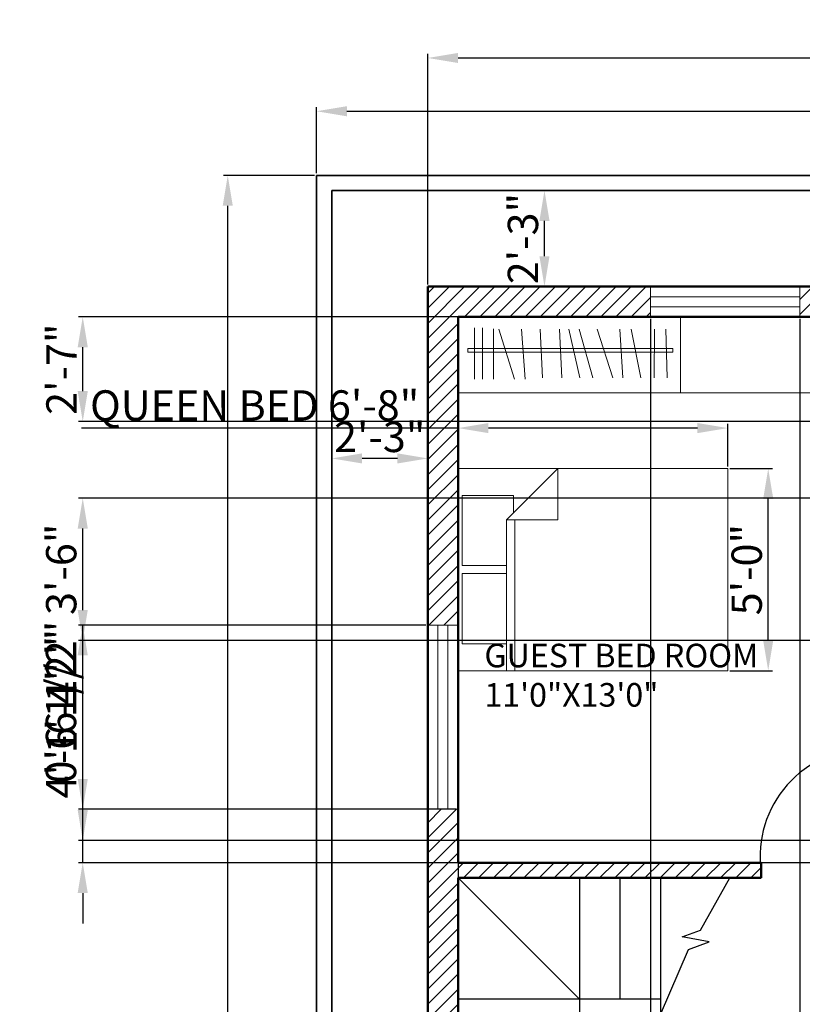
# Model space of a CAD drawing. Units: inches. Extents: x 53662 to 54269, y 37303 to 38048.
# Tile 5 of 6: x 53662 to 53894, y 37749 to 38041. Entities that reach past the tile are written whole.
import ezdxf

# ---------------------------------------------------------------- set-up
doc = ezdxf.new("R2010")
doc.units = ezdxf.units.IN
for name, color, linetype, lineweight in [('A-ANNO-DIMS', 2, 'Continuous', 18), ('A-AREA-IDEN', 7, 'Continuous', 25), ('A-DOOR', 3, 'Continuous', 25), ('A-FLOR-CASE', 8, 'Continuous', 18), ('A-FLOR-STRS', 7, 'Continuous', 25), ('A-FURN', 8, 'Continuous', 18), ('A-GLAZ', 4, 'Continuous', 18), ('A-WALL', 7, 'Continuous', 50), ('C-PROP', 7, 'Continuous', 35)]:
    doc.layers.add(name, color=color, linetype=linetype, lineweight=lineweight)
doc.layers.add('A-WALL-PATT', color=244, linetype='Continuous', lineweight=13, true_color=0x991b1e)
doc.styles.get("Standard").update_dxf_attribs({"font": 'arial.ttf'})
doc.dimstyles.new('ISO-25', dxfattribs={"dimtxt": 9, "dimasz": 9, "dimexe": 1.25, "dimexo": 0.625, "dimtad": 1, "dimdec": 1, "dimrnd": 9, "dimlunit": 3, "dimtxsty": 'Standard', "dimcen": 2.5, "dimadec": 0, "dimazin": 0, "dimtfac": 1, "dimtdec": 1, "dimtmove": 0, "dimatfit": 3, "dimfxl": 1, "dimarcsym": 0})

# ---------------------------------------------------------------- blocks, each defined once
blk = doc.blocks.new('Bed - Queen')
for p, q in [((0, -80.00003), (0, 0)), ((0, 0), (59.99999, 0)), ((59.99999, 0), (59.99999, -80.00003)), ((7.99999, -1.2), (28.79998, -1.2)), ((7.99999, -14.4), (7.99999, -1.2)), ((28.79998, -1.2), (28.79998, -14.4)), ((31.19999, -1.2), (51.99999, -1.2)), ((31.19999, -14.4), (31.19999, -1.2)), ((51.99999, -1.2), (51.99999, -16.4)), ((0, -14.4), (44.8, -14.4)), ((59.99999, -29.6), (44.8, -14.4)), ((44.8, -14.4), (44.8, -29.6)), ((44.8, -16.8), (0, -16.8)), ((51.99999, -16.4), (46.79936, -16.4)), ((44.8, -29.6), (59.99999, -29.6)), ((59.99999, -80.00003), (0, -80.00003))]:
    blk.add_line(p, q)
blk = doc.blocks.new('*D10')
at = {"layer": 'A-ANNO-DIMS', "color": 0, "lineweight": -2, "transparency": 16777216}
for p, q in [((53783.74, 37990.36), (53818.98, 37990.36)), ((53817.73, 37970.86), (53817.73, 37981.36)), ((53783.74, 37961.86), (53818.98, 37961.86))]:
    blk.add_line(p, q, dxfattribs=at)
at = {"layer": 'A-ANNO-DIMS', "color": 0, "transparency": 16777216}
for points in [[(53816.23, 37981.36), (53819.23, 37981.36), (53817.73, 37990.36)], [(53816.23, 37970.86), (53819.23, 37970.86), (53817.73, 37961.86)]]:
    blk.add_solid(points, dxfattribs=at)
at = {"layer": 'Defpoints', "color": 0, "transparency": 16777216}
for p in [(53783.11, 37990.36), (53817.73, 37990.36), (53783.11, 37961.86)]:
    blk.add_point(p, dxfattribs=at)
at = {"layer": 'A-ANNO-DIMS', "color": 0, "transparency": 16777216, "insert": (53812.51, 37976.11), "char_height": 9, "attachment_point": 5, "rotation": 90}
blk.add_mtext('2\'-3"', dxfattribs=at)
blk = doc.blocks.new('*D12')
at = {"layer": 'A-ANNO-DIMS', "color": 0, "lineweight": -2, "transparency": 16777216}
for p, q in [((53754.61, 37961.24), (53754.61, 37909.61)), ((53783.11, 37961.24), (53783.11, 37909.61)), ((53774.11, 37910.86), (53763.61, 37910.86))]:
    blk.add_line(p, q, dxfattribs=at)
at = {"layer": 'A-ANNO-DIMS', "color": 0, "transparency": 16777216}
for points in [[(53763.61, 37912.36), (53763.61, 37909.36), (53754.61, 37910.86)], [(53774.11, 37912.36), (53774.11, 37909.36), (53783.11, 37910.86)]]:
    blk.add_solid(points, dxfattribs=at)
at = {"layer": 'Defpoints', "color": 0, "transparency": 16777216}
for p in [(53754.61, 37961.86), (53783.11, 37961.86), (53754.61, 37910.86)]:
    blk.add_point(p, dxfattribs=at)
at = {"layer": 'A-ANNO-DIMS', "color": 0, "transparency": 16777216, "insert": (53768.86, 37916.08), "char_height": 9, "attachment_point": 5}
blk.add_mtext('2\'-3"', dxfattribs=at)
blk = doc.blocks.new('*D13')
at = {"layer": 'A-ANNO-DIMS', "color": 0, "lineweight": -2, "transparency": 16777216}
for p, q in [((53749.49, 37994.86), (53722.52, 37994.86)), ((53723.77, 37427.86), (53723.77, 37985.86)), ((53749.49, 37418.86), (53722.52, 37418.86))]:
    blk.add_line(p, q, dxfattribs=at)
at = {"layer": 'A-ANNO-DIMS', "color": 0, "transparency": 16777216}
for points in [[(53722.27, 37985.86), (53725.27, 37985.86), (53723.77, 37994.86)], [(53722.27, 37427.86), (53725.27, 37427.86), (53723.77, 37418.86)]]:
    blk.add_solid(points, dxfattribs=at)
at = {"layer": 'Defpoints', "color": 0, "transparency": 16777216}
for p in [(53723.77, 37994.86), (53750.11, 37994.86), (53750.11, 37418.86)]:
    blk.add_point(p, dxfattribs=at)
at = {"layer": 'A-ANNO-DIMS', "color": 0, "transparency": 16777216, "insert": (53718.55, 37706.86), "char_height": 9, "attachment_point": 5, "rotation": 90}
blk.add_mtext("48'", dxfattribs=at)
blk = doc.blocks.new('*D14')
at = {"layer": 'A-ANNO-DIMS', "color": 0, "lineweight": -2, "transparency": 16777216}
for p, q in [((53750.11, 37995.49), (53750.11, 38015.14)), ((54182.11, 37995.49), (54182.11, 38015.14)), ((53759.11, 38013.89), (54173.11, 38013.89))]:
    blk.add_line(p, q, dxfattribs=at)
at = {"layer": 'A-ANNO-DIMS', "color": 0, "transparency": 16777216}
for points in [[(53759.11, 38015.39), (53759.11, 38012.39), (53750.11, 38013.89)], [(54173.11, 38015.39), (54173.11, 38012.39), (54182.11, 38013.89)]]:
    blk.add_solid(points, dxfattribs=at)
at = {"layer": 'Defpoints', "color": 0, "transparency": 16777216}
for p in [(54182.11, 38013.89), (53750.11, 37994.86), (54182.11, 37994.86)]:
    blk.add_point(p, dxfattribs=at)
at = {"layer": 'A-ANNO-DIMS', "color": 0, "transparency": 16777216, "insert": (53966.11, 38019.11), "char_height": 9, "attachment_point": 5}
blk.add_mtext("36'", dxfattribs=at)
blk = doc.blocks.new('*D28')
at = {"layer": 'A-ANNO-DIMS', "color": 0, "lineweight": -2, "transparency": 16777216}
for p, q in [((53792.11, 37908.49), (53792.11, 37921.11)), ((53872.11, 37908.49), (53872.11, 37921.11)), ((53792.11, 37919.86), (53680.41, 37919.86)), ((53863.11, 37919.86), (53801.11, 37919.86))]:
    blk.add_line(p, q, dxfattribs=at)
at = {"layer": 'A-ANNO-DIMS', "color": 0, "transparency": 16777216}
for points in [[(53801.11, 37921.36), (53801.11, 37918.36), (53792.11, 37919.86)], [(53863.11, 37921.36), (53863.11, 37918.36), (53872.11, 37919.86)]]:
    blk.add_solid(points, dxfattribs=at)
at = {"layer": 'Defpoints', "color": 0, "transparency": 16777216}
for p in [(53792.11, 37919.86), (53792.11, 37907.86), (53872.11, 37907.86)]:
    blk.add_point(p, dxfattribs=at)
at = {"layer": 'A-ANNO-DIMS', "color": 0, "transparency": 16777216, "insert": (53731.76, 37925.41), "char_height": 9, "attachment_point": 5}
blk.add_mtext('QUEEN BED 6\'-8"', dxfattribs=at)
blk = doc.blocks.new('*D29')
at = {"layer": 'A-ANNO-DIMS', "color": 0, "lineweight": -2, "transparency": 16777216}
for p, q in [((53872.74, 37907.86), (53885.36, 37907.86)), ((53884.11, 37856.86), (53884.11, 37898.86)), ((53872.74, 37847.86), (53885.36, 37847.86))]:
    blk.add_line(p, q, dxfattribs=at)
at = {"layer": 'A-ANNO-DIMS', "color": 0, "transparency": 16777216}
for points in [[(53882.61, 37898.86), (53885.61, 37898.86), (53884.11, 37907.86)], [(53882.61, 37856.86), (53885.61, 37856.86), (53884.11, 37847.86)]]:
    blk.add_solid(points, dxfattribs=at)
at = {"layer": 'Defpoints', "color": 0, "transparency": 16777216}
for p in [(53872.11, 37907.86), (53884.11, 37907.86), (53872.11, 37847.86)]:
    blk.add_point(p, dxfattribs=at)
at = {"layer": 'A-ANNO-DIMS', "color": 0, "transparency": 16777216, "insert": (53878.89, 37877.86), "char_height": 9, "attachment_point": 5, "rotation": 90}
blk.add_mtext('5\'-0"', dxfattribs=at)
blk = doc.blocks.new('*D40')
at = {"layer": 'A-ANNO-DIMS', "color": 0, "lineweight": -2, "transparency": 16777216}
for p, q in [((53920.32, 37824.61), (53920.32, 37973.07)), ((53915.54, 37824.61), (53921.57, 37824.61)), ((53920.32, 37797.61), (53920.32, 37815.61)), ((53915.54, 37788.61), (53921.57, 37788.61))]:
    blk.add_line(p, q, dxfattribs=at)
at = {"layer": 'A-ANNO-DIMS', "color": 0, "transparency": 16777216}
for points in [[(53918.82, 37815.61), (53921.82, 37815.61), (53920.32, 37824.61)], [(53918.82, 37797.61), (53921.82, 37797.61), (53920.32, 37788.61)]]:
    blk.add_solid(points, dxfattribs=at)
at = {"layer": 'Defpoints', "color": 0, "transparency": 16777216}
for p in [(53914.92, 37824.61), (53920.32, 37824.61), (53914.92, 37788.61)]:
    blk.add_point(p, dxfattribs=at)
at = {"layer": 'A-ANNO-DIMS', "color": 0, "transparency": 16777216, "insert": (53915.03, 37903.34), "char_height": 9, "attachment_point": 5, "rotation": 90}
blk.add_mtext('ROOM DOOR 3\'-0" TYP.', dxfattribs=at)
blk = doc.blocks.new('*D50')
at = {"layer": 'A-ANNO-DIMS', "color": 0, "lineweight": -2, "transparency": 16777216}
for p, q in [((53783.11, 37962.49), (53783.11, 38030.96)), ((53792.11, 38029.71), (54137.11, 38029.71)), ((54146.11, 37962.49), (54146.11, 38030.96))]:
    blk.add_line(p, q, dxfattribs=at)
at = {"layer": 'A-ANNO-DIMS', "color": 0, "transparency": 16777216}
for points in [[(53792.11, 38031.21), (53792.11, 38028.21), (53783.11, 38029.71)], [(54137.11, 38031.21), (54137.11, 38028.21), (54146.11, 38029.71)]]:
    blk.add_solid(points, dxfattribs=at)
at = {"layer": 'Defpoints', "color": 0, "transparency": 16777216}
for p in [(54146.11, 38029.71), (53783.11, 37961.86), (54146.11, 37961.86)]:
    blk.add_point(p, dxfattribs=at)
at = {"layer": 'A-ANNO-DIMS', "color": 0, "transparency": 16777216, "insert": (53964.61, 38034.93), "char_height": 9, "attachment_point": 5}
blk.add_mtext('30\'-3"', dxfattribs=at)
blk = doc.blocks.new('*D54')
at = {"layer": 'A-ANNO-DIMS', "color": 0, "lineweight": -2, "transparency": 16777216}
for p, q in [((53792.11, 37952.24), (53792.11, 37309.49)), ((53849.2, 37952.24), (53849.2, 37309.49)), ((53801.11, 37310.74), (53840.2, 37310.74))]:
    blk.add_line(p, q, dxfattribs=at)
at = {"layer": 'A-ANNO-DIMS', "color": 0, "transparency": 16777216}
for points in [[(53801.11, 37312.24), (53801.11, 37309.24), (53792.11, 37310.74)], [(53840.2, 37312.24), (53840.2, 37309.24), (53849.2, 37310.74)]]:
    blk.add_solid(points, dxfattribs=at)
at = {"layer": 'Defpoints', "color": 0, "transparency": 16777216}
for p in [(53792.11, 37952.86), (53849.2, 37952.86), (53849.2, 37310.74)]:
    blk.add_point(p, dxfattribs=at)
at = {"layer": 'A-ANNO-DIMS', "color": 0, "transparency": 16777216, "insert": (53820.66, 37315.96), "char_height": 9, "attachment_point": 5}
blk.add_mtext('4\'-9"', dxfattribs=at)
blk = doc.blocks.new('*D55')
at = {"layer": 'A-ANNO-DIMS', "color": 0, "lineweight": -2, "transparency": 16777216}
for p, q in [((53849.2, 37952.24), (53849.2, 37309.49)), ((53893.52, 37952.24), (53893.52, 37309.49)), ((53858.2, 37310.74), (53884.52, 37310.74)), ((53893.52, 37310.74), (53948.66, 37310.74))]:
    blk.add_line(p, q, dxfattribs=at)
at = {"layer": 'A-ANNO-DIMS', "color": 0, "transparency": 16777216}
for points in [[(53858.2, 37312.24), (53858.2, 37309.24), (53849.2, 37310.74)], [(53884.52, 37312.24), (53884.52, 37309.24), (53893.52, 37310.74)]]:
    blk.add_solid(points, dxfattribs=at)
at = {"layer": 'Defpoints', "color": 0, "transparency": 16777216}
for p in [(53849.2, 37952.86), (53893.52, 37952.86), (53893.52, 37310.74)]:
    blk.add_point(p, dxfattribs=at)
at = {"layer": 'A-ANNO-DIMS', "color": 0, "transparency": 16777216, "insert": (53925.59, 37316.02), "char_height": 9, "attachment_point": 5}
blk.add_mtext('3\'-8 1/2"', dxfattribs=at)
blk = doc.blocks.new('*D62')
at = {"layer": 'A-ANNO-DIMS', "color": 0, "lineweight": -2, "transparency": 16777216}
for p, q in [((53680.75, 37815.76), (53680.75, 37849.09)), ((53791.49, 37806.76), (53679.5, 37806.76)), ((53680.75, 37790.86), (53680.75, 37806.76)), ((53791.49, 37790.86), (53679.5, 37790.86)), ((53680.75, 37781.86), (53680.75, 37772.86))]:
    blk.add_line(p, q, dxfattribs=at)
at = {"layer": 'A-ANNO-DIMS', "color": 0, "transparency": 16777216}
for points in [[(53679.25, 37815.76), (53682.25, 37815.76), (53680.75, 37806.76)], [(53679.25, 37781.86), (53682.25, 37781.86), (53680.75, 37790.86)]]:
    blk.add_solid(points, dxfattribs=at)
at = {"layer": 'Defpoints', "color": 0, "transparency": 16777216}
for p in [(53680.75, 37806.76), (53792.11, 37806.76), (53792.11, 37790.86)]:
    blk.add_point(p, dxfattribs=at)
at = {"layer": 'A-ANNO-DIMS', "color": 0, "transparency": 16777216, "insert": (53675.61, 37836.93), "char_height": 9, "attachment_point": 5, "rotation": 90}
blk.add_mtext('1\'-4"', dxfattribs=at)
blk = doc.blocks.new('*D63')
at = {"layer": 'A-ANNO-DIMS', "color": 0, "lineweight": -2, "transparency": 16777216}
for p, q in [((53782.49, 37861.42), (53679.5, 37861.42)), ((53680.75, 37815.76), (53680.75, 37852.42)), ((53782.49, 37806.76), (53679.5, 37806.76))]:
    blk.add_line(p, q, dxfattribs=at)
at = {"layer": 'A-ANNO-DIMS', "color": 0, "transparency": 16777216}
for points in [[(53679.25, 37852.42), (53682.25, 37852.42), (53680.75, 37861.42)], [(53679.25, 37815.76), (53682.25, 37815.76), (53680.75, 37806.76)]]:
    blk.add_solid(points, dxfattribs=at)
at = {"layer": 'Defpoints', "color": 0, "transparency": 16777216}
for p in [(53680.75, 37861.42), (53783.11, 37861.42), (53783.11, 37806.76)]:
    blk.add_point(p, dxfattribs=at)
at = {"layer": 'A-ANNO-DIMS', "color": 0, "transparency": 16777216, "insert": (53675.47, 37834.09), "char_height": 9, "attachment_point": 5, "rotation": 90}
blk.add_mtext('4\'-6 1/2"', dxfattribs=at)
blk = doc.blocks.new('*D72')
at = {"layer": 'A-ANNO-DIMS', "color": 0, "lineweight": -2, "transparency": 16777216}
for p, q in [((53981.99, 37899.06), (53679.5, 37899.06)), ((53680.75, 37865.86), (53680.75, 37890.06)), ((53981.99, 37856.86), (53679.5, 37856.86))]:
    blk.add_line(p, q, dxfattribs=at)
at = {"layer": 'A-ANNO-DIMS', "color": 0, "transparency": 16777216}
for points in [[(53679.25, 37890.06), (53682.25, 37890.06), (53680.75, 37899.06)], [(53679.25, 37865.86), (53682.25, 37865.86), (53680.75, 37856.86)]]:
    blk.add_solid(points, dxfattribs=at)
at = {"layer": 'Defpoints', "color": 0, "transparency": 16777216}
for p in [(53680.75, 37899.06), (53982.61, 37899.06), (53982.61, 37856.86)]:
    blk.add_point(p, dxfattribs=at)
at = {"layer": 'A-ANNO-DIMS', "color": 0, "transparency": 16777216, "insert": (53675.53, 37877.96), "char_height": 9, "attachment_point": 5, "rotation": 90}
blk.add_mtext('3\'-6"', dxfattribs=at)
blk = doc.blocks.new('*D73')
at = {"layer": 'A-ANNO-DIMS', "color": 0, "lineweight": -2, "transparency": 16777216}
for p, q in [((53927.99, 37952.86), (53679.5, 37952.86)), ((53680.75, 37930.83), (53680.75, 37943.86)), ((53927.99, 37921.83), (53679.5, 37921.83))]:
    blk.add_line(p, q, dxfattribs=at)
at = {"layer": 'A-ANNO-DIMS', "color": 0, "transparency": 16777216}
for points in [[(53679.25, 37943.86), (53682.25, 37943.86), (53680.75, 37952.86)], [(53679.25, 37930.83), (53682.25, 37930.83), (53680.75, 37921.83)]]:
    blk.add_solid(points, dxfattribs=at)
at = {"layer": 'Defpoints', "color": 0, "transparency": 16777216}
for p in [(53680.75, 37952.86), (53928.61, 37952.86), (53928.61, 37921.83)]:
    blk.add_point(p, dxfattribs=at)
at = {"layer": 'A-ANNO-DIMS', "color": 0, "transparency": 16777216, "insert": (53675.61, 37937.35), "char_height": 9, "attachment_point": 5, "rotation": 90}
blk.add_mtext('2\'-7"', dxfattribs=at)
blk = doc.blocks.new('*D74')
at = {"layer": 'A-ANNO-DIMS', "color": 0, "lineweight": -2, "transparency": 16777216}
for p, q in [((53680.75, 37806.48), (53680.75, 37861.62)), ((53981.99, 37797.48), (53679.5, 37797.48)), ((53680.75, 37790.86), (53680.75, 37797.48)), ((53981.99, 37790.86), (53679.5, 37790.86)), ((53680.75, 37781.86), (53680.75, 37772.86))]:
    blk.add_line(p, q, dxfattribs=at)
at = {"layer": 'A-ANNO-DIMS', "color": 0, "transparency": 16777216}
for points in [[(53679.25, 37806.48), (53682.25, 37806.48), (53680.75, 37797.48)], [(53679.25, 37781.86), (53682.25, 37781.86), (53680.75, 37790.86)]]:
    blk.add_solid(points, dxfattribs=at)
at = {"layer": 'Defpoints', "color": 0, "transparency": 16777216}
for p in [(53680.75, 37797.48), (53982.61, 37797.48), (53982.61, 37790.86)]:
    blk.add_point(p, dxfattribs=at)
at = {"layer": 'A-ANNO-DIMS', "color": 0, "transparency": 16777216, "insert": (53675.47, 37838.55), "char_height": 9, "attachment_point": 5, "rotation": 90}
blk.add_mtext('0\'-6 1/2"', dxfattribs=at)

msp = doc.modelspace()

# ---------------------------------------------------------------- hatches: boundary and pattern name
at = {"layer": 'A-WALL-PATT'}
h = msp.add_hatch(dxfattribs=at)
h.set_pattern_fill('ANSI31', color=256)
h.paths.add_polyline_path([(53792.11, 37952.86), (53849.2, 37952.86), (53849.2, 37961.86), (53783.11, 37961.86), (53783.11, 37861.42), (53792.11, 37861.42)])
h.paths.add_polyline_path([(53940.97, 37961.86), (53893.52, 37961.86), (53893.52, 37952.86), (53924.11, 37952.86), (53924.11, 37921.83), (53926.36, 37921.83, -0.026334), (53928.61, 37921.99), (53928.61, 37930.37), (53928.61, 37952.86), (53940.97, 37952.86)])
h.paths.add_polyline_path([(53792.11, 37786.36), (53882.05, 37786.36), (53882.05, 37788.61, -0.017862), (53881.82, 37790.86), (53792.11, 37790.86), (53792.11, 37806.76), (53783.11, 37806.76), (53783.11, 37732.86), (53792.11, 37732.86)])
h.paths.add_polyline_path([(53792.11, 37672.86), (53783.11, 37672.86), (53783.11, 37615.86), (53804.11, 37615.86), (53804.11, 37599.43), (53813.11, 37599.43), (53813.11, 37620.36), (53922.61, 37620.36), (53922.61, 37624.86), (53792.11, 37624.86)])
h.paths.add_polyline_path([(53978.11, 37572.86), (53927.11, 37572.86), (53927.11, 37620.36), (53922.61, 37620.36), (53922.61, 37568.36), (53978.11, 37568.36)])
h.paths.add_polyline_path([(53927.11, 37624.86), (53922.61, 37624.86), (53922.61, 37620.36), (53927.11, 37620.36)])
h.paths.add_polyline_path([(53987.11, 37615.86), (54079.03, 37615.86), (54079.03, 37624.86), (53978.11, 37624.86), (53978.11, 37471.86), (53926.17, 37471.86), (53926.17, 37462.86), (53987.11, 37462.86)])
h.paths.add_polyline_path([(53813.11, 37561.58), (53804.11, 37561.58), (53804.11, 37471.86), (53783.11, 37471.86), (53783.11, 37462.86), (53873.85, 37462.86), (53873.85, 37471.86), (53813.11, 37471.86)])
h.paths.add_polyline_path([(54146.11, 37687.42), (54137.11, 37687.42), (54137.11, 37624.86), (54128.99, 37624.86), (54128.99, 37615.86), (54146.11, 37615.86)])
h.paths.add_polyline_path([(54146.11, 37813.18), (54137.11, 37813.18), (54137.11, 37747.89), (54146.11, 37747.89)])
h.paths.add_polyline_path([(54146.11, 37961.86), (54107.27, 37961.86), (54107.27, 37952.86), (54137.11, 37952.86), (54137.11, 37884.55), (54146.11, 37884.55)])
h.paths.add_polyline_path([(54022.12, 37961.86), (53964.61, 37961.86), (53964.61, 37952.86), (53982.61, 37952.86), (53982.61, 37822.8), (53987.11, 37822.8), (53987.11, 37952.86), (54022.12, 37952.86)])
h.paths.add_polyline_path([(53928.61, 37899.06), (53924.11, 37899.06), (53924.11, 37790.86), (53914.92, 37790.86), (53914.92, 37786.36), (53987.11, 37786.36), (53987.11, 37797.48), (53982.61, 37797.48), (53982.61, 37790.86), (53928.61, 37790.86), (53928.61, 37801.6, -0.072813), (53928.13, 37805.9, -0.05664), (53928.61, 37809.23)])

# ---------------------------------------------------------------- linework, layer by layer
at = {"layer": 'A-DOOR'}
msp.add_arc((53913.42, 37792.95), 31.67, 89.0952, 187.8757, dxfattribs=at)
at = {"layer": 'A-FLOR-CASE'}
for p, q in [((53858.11, 37952.86), (53858.11, 37930.37)), ((53796.95, 37949.61), (53796.95, 37934.43)), ((53799.32, 37949.61), (53799.32, 37934.43)), ((53802.59, 37949.36), (53802.59, 37934.43)), ((53804.2, 37949.24), (53808.83, 37934.43)), ((53810.92, 37949.24), (53812.05, 37934.43)), ((53816.45, 37949.24), (53817.18, 37934.82)), ((53822.2, 37949.24), (53822.85, 37934.82)), ((53824.98, 37949.24), (53828.2, 37934.82)), ((53828.05, 37949.24), (53832.04, 37934.82)), ((53833.37, 37949.24), (53837.97, 37934.82)), ((53840.07, 37949.24), (53840.99, 37934.82)), ((53843.47, 37949.24), (53846.35, 37934.78)), ((53850.37, 37949.24), (53850.29, 37934.78)), ((53853.73, 37949.22), (53854.14, 37934.78)), ((53924.11, 37930.37), (53792.11, 37930.37))]:
    msp.add_line(p, q, dxfattribs=at)
msp.add_lwpolyline([(53794.96, 37943.44), (53855.79, 37943.44), (53855.79, 37942.39), (53794.96, 37942.39)], close=True, dxfattribs=at)
at = {"layer": 'A-FLOR-STRS'}
for p, q in [((53828.11, 37750.36), (53792.11, 37786.36)), ((53828.11, 37786.36), (53828.11, 37624.86)), ((53840.11, 37786.36), (53840.11, 37750.36)), ((53852.11, 37786.36), (53852.11, 37745.86)), ((53863.98, 37770.81), (53872.73, 37786.36)), ((53858.57, 37768.83), (53863.98, 37770.81)), ((53866.54, 37767.43), (53858.57, 37768.83)), ((53860.44, 37765.15), (53866.54, 37767.43)), ((53852.11, 37745.86), (53860.44, 37765.15)), ((53852.11, 37750.36), (53792.11, 37750.36))]:
    msp.add_line(p, q, dxfattribs=at)
at = {"layer": 'A-GLAZ'}
for p, q in [((53849.2, 37961.86), (53849.2, 37952.86)), ((53893.52, 37961.86), (53893.52, 37952.86)), ((53893.52, 37958.86), (53849.2, 37958.86)), ((53893.52, 37955.86), (53849.2, 37955.86)), ((53792.11, 37861.42), (53783.11, 37861.42)), ((53786.11, 37861.42), (53786.11, 37806.76)), ((53789.11, 37861.42), (53789.11, 37806.76)), ((53792.11, 37806.76), (53783.11, 37806.76))]:
    msp.add_line(p, q, dxfattribs=at)
at = {"layer": 'A-WALL'}
for p, q in [((54146.11, 37961.86), (53783.11, 37961.86)), ((53783.11, 37961.86), (53783.11, 37615.86)), ((53792.11, 37952.86), (53792.11, 37790.86)), ((53924.11, 37952.86), (53792.11, 37952.86)), ((53882.05, 37790.86), (53792.11, 37790.86)), ((53882.05, 37790.86), (53882.05, 37786.36)), ((53882.05, 37786.36), (53792.11, 37786.36)), ((53792.11, 37786.36), (53792.11, 37624.86))]:
    msp.add_line(p, q, dxfattribs=at)
at = {"layer": 'C-PROP'}
for p, q in [((54182.11, 37994.86), (53750.11, 37994.86)), ((53750.11, 37994.86), (53750.11, 37615.86)), ((54177.61, 37990.36), (53754.61, 37990.36)), ((53754.61, 37990.36), (53754.61, 37615.86))]:
    msp.add_line(p, q, dxfattribs=at)

# ---------------------------------------------------------------- block references
at = {"layer": 'A-FURN', "rotation": 90}
msp.add_blockref('Bed - Queen', (53792.11, 37847.86), dxfattribs=at)

# ---------------------------------------------------------------- texts
at = {"layer": 'A-AREA-IDEN', "insert": (53799.91, 37855.86), "char_height": 7, "attachment_point": 1}
msp.add_mtext_dynamic_manual_height_columns('GUEST BED ROOM\\P11\'0"X13\'0"', width=119.3618, gutter_width=12.5, heights=[0], dxfattribs=at)

# ---------------------------------------------------------------- dimensions: what is measured, and where the dimension line sits
at = {"layer": 'A-ANNO-DIMS'}
for base, p1, p2, override, picture, middle in [((54146.11, 38029.71), (53783.11, 37961.86), (54146.11, 37961.86), {"dimdec": 1, "dimlfac": 1, "dimrnd": 0, "dimzin": 1, "dimdsep": 46, "dimlunit": 4, "dimfrac": 2}, '*D50', (53964.61, 38034.93)), ((54182.11, 38013.89), (53750.11, 37994.86), (54182.11, 37994.86), {"dimclrd": 0, "dimclre": 0, "dimclrt": 0}, '*D14', (53966.11, 38019.11)), ((53754.61, 37910.86), (53783.11, 37961.86), (53754.61, 37961.86), {"dimclrd": 0, "dimclre": 0, "dimclrt": 0}, '*D12', (53768.86, 37916.08)), ((53849.2, 37310.74), (53792.11, 37952.86), (53849.2, 37952.86), {"dimdec": 1, "dimlfac": 1, "dimrnd": 0, "dimzin": 1, "dimdsep": 46, "dimlunit": 4, "dimfrac": 2}, '*D54', (53820.66, 37315.96)), ((53893.52, 37310.74), (53849.2, 37952.86), (53893.52, 37952.86), {"dimdec": 1, "dimlfac": 1, "dimrnd": 0, "dimzin": 1, "dimdsep": 46, "dimlunit": 4, "dimfrac": 2}, '*D55', (53925.59, 37316.02))]:
    dim = msp.add_linear_dim(base=base, p1=p1, p2=p2, dimstyle='ISO-25', override=override, dxfattribs=at)
    dim.commit()
    dim.dimension.update_dxf_attribs({"geometry": picture, "text_midpoint": middle})
for base, p1, p2, override, picture, middle in [((53723.77, 37994.86), (53750.11, 37418.86), (53750.11, 37994.86), {"dimclrd": 0, "dimclre": 0, "dimclrt": 0}, '*D13', (53718.55, 37706.86)), ((53817.73, 37990.36), (53783.11, 37961.86), (53783.11, 37990.36), {"dimclrd": 0, "dimclre": 0, "dimclrt": 0}, '*D10', (53812.51, 37976.11)), ((53680.75, 37952.86), (53928.61, 37921.83), (53928.61, 37952.86), {"dimdec": 1, "dimlfac": 1, "dimrnd": 0, "dimzin": 1, "dimdsep": 46, "dimlunit": 4, "dimfrac": 2}, '*D73', (53675.61, 37937.35)), ((53884.11, 37907.86), (53872.11, 37847.86), (53872.11, 37907.86), {"dimdec": 1, "dimlfac": 1, "dimrnd": 0, "dimzin": 1, "dimdsep": 46, "dimlunit": 4, "dimfrac": 2}, '*D29', (53878.89, 37877.86)), ((53680.75, 37899.06), (53982.61, 37856.86), (53982.61, 37899.06), {"dimdec": 1, "dimlfac": 1, "dimrnd": 0, "dimzin": 1, "dimdsep": 46, "dimlunit": 4, "dimfrac": 2}, '*D72', (53675.53, 37877.96)), ((53680.75, 37797.48), (53982.61, 37790.86), (53982.61, 37797.48), {"dimdec": 1, "dimlfac": 1, "dimrnd": 0, "dimzin": 1, "dimdsep": 46, "dimlunit": 4, "dimfrac": 2}, '*D74', (53675.47, 37838.55)), ((53680.75, 37861.42), (53783.11, 37806.76), (53783.11, 37861.42), {"dimdec": 1, "dimlfac": 1, "dimrnd": 0, "dimzin": 1, "dimdsep": 46, "dimlunit": 4, "dimfrac": 2}, '*D63', (53675.47, 37834.09)), ((53680.75, 37806.76), (53792.11, 37790.86), (53792.11, 37806.76), {"dimdec": 1, "dimlfac": 1, "dimrnd": 0, "dimzin": 1, "dimdsep": 46, "dimlunit": 4, "dimfrac": 2}, '*D62', (53675.61, 37836.93))]:
    dim = msp.add_linear_dim(base=base, p1=p1, p2=p2, angle=90, dimstyle='ISO-25', override=override, dxfattribs=at)
    dim.commit()
    dim.dimension.update_dxf_attribs({"geometry": picture, "text_midpoint": middle})
for base, p1, p2, angle, text, picture, middle in [((53920.32, 37824.61), (53914.92, 37788.61), (53914.92, 37824.61), 90, 'ROOM DOOR <> TYP.', '*D40', (53915.03, 37903.34)), ((53792.11, 37919.86), (53872.11, 37907.86), (53792.11, 37907.86), 180, 'QUEEN BED <>', '*D28', (53731.76, 37925.41))]:
    dim = msp.add_linear_dim(base=base, p1=p1, p2=p2, angle=angle, text=text, dimstyle='ISO-25', override={"dimdec": 1, "dimlfac": 1, "dimrnd": 0, "dimzin": 1, "dimdsep": 46, "dimlunit": 4, "dimfrac": 2}, dxfattribs=at)
    dim.commit()
    dim.dimension.update_dxf_attribs({"geometry": picture, "text_midpoint": middle})

doc.saveas('drawing.dxf')
